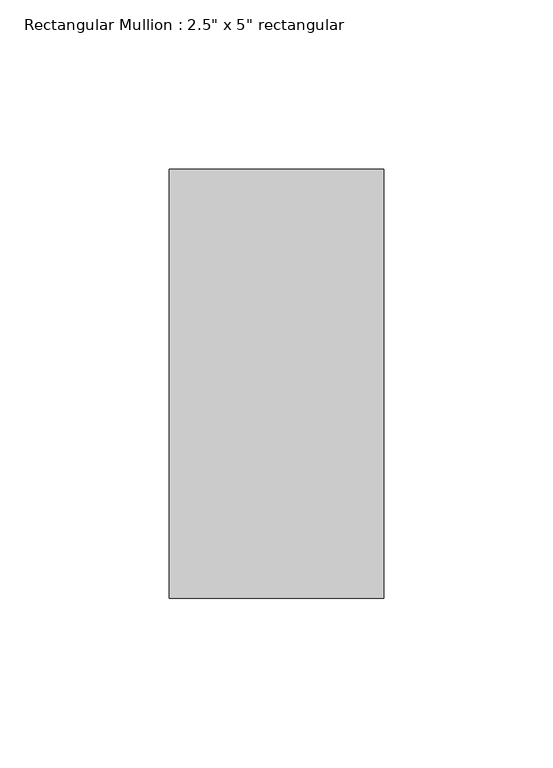
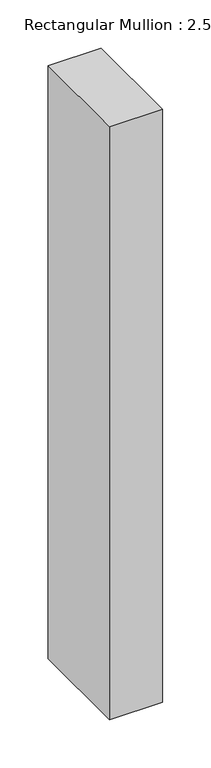
"""IFC4 building model written with IfcOpenShell, lengths in millimetres: member geometry."""

from ifc_helpers import new_model, si_unit, frame, origin, place, context, project, spatial, polyline, outline, extrude, source, transform, mapped, element, save


def member_9d02be77(model_context):
    return source(origin(), model_context, "Body", "SweptSolid", [
        extrude(outline(polyline([(0.0, 63.5), (0.0, -63.5), (-63.5, -63.5), (-63.5, 63.5), (0.0, 63.5)])), frame((0.0, 0.0, -749.3), z_axis=(0.0, 0.0, 1.0), x_axis=(1.0, 0.0, 0.0)), (0.0, 0.0, 1.0), 749.3),
    ])


if __name__ == "__main__":
    model = new_model("IFC4")
    model_context = context("Model", 3, world=origin())
    ifc_project = project(units=[si_unit("LENGTHUNIT", "METRE", prefix="MILLI")], contexts=[model_context])
    site = spatial("IfcSite", under=ifc_project)
    building = spatial("IfcBuilding", under=site)
    placement = place(None, origin())
    member_shape = member_9d02be77(model_context)
    element("IfcMember", 1, ObjectType="Rectangular Mullion : 2.5\" x 5\" rectangular", at=placement, inside=building, context=model_context, shape_type="MappedRepresentation", body=[
        mapped(member_shape, transform((0.0, 0.0, 0.0), x_axis=(1.0, 0.0, 0.0), y_axis=(0.0, 1.0, 0.0), z_axis=(0.0, 0.0, 1.0))),
    ])
    save(model, "model.ifc")

# Revit data of these elements
# Type "Rectangular Mullion : 2.5\" x 5\" rectangular"
#   built-in parameter 1007304 = 0.416667 (stored number, unit not read)
#   built-in parameter 1007301 = 0.104167 (stored number, unit not read)
#   built-in parameter 1007300 = 0.104167 (stored number, unit not read)
